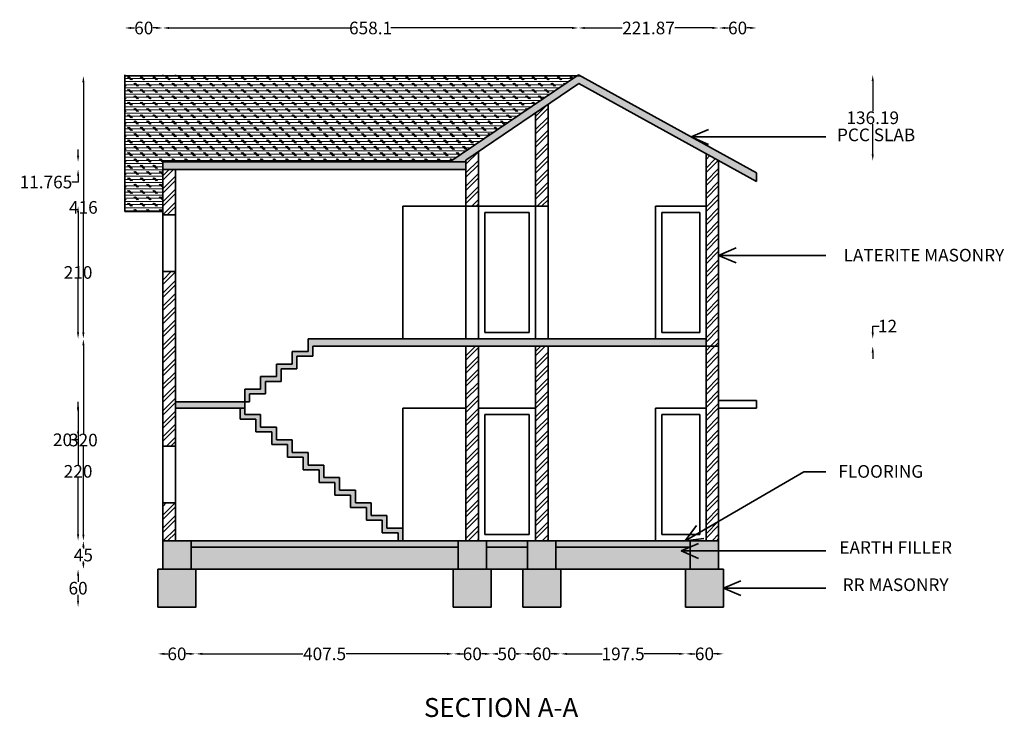
# Model space of a CAD drawing. Units: centimetres. Extents: x 10444 to 13814, y 8288 to 11191.
# Tile 7 of 9: x 12167 to 13725, y 8288 to 9393. Entities that reach past the tile are written whole.
import ezdxf

# ---------------------------------------------------------------- set-up
doc = ezdxf.new("R2010")
doc.units = ezdxf.units.CM
doc.header["$MEASUREMENT"] = 0
for name, color, linetype, lineweight in [('A-ANNO-DIMS', 2, 'Continuous', 18), ('A-ANNO-TEXT', 7, 'Continuous', 25), ('A-SECT', 7, 'Continuous', 35), ('A-SECT-PATT', 8, 'Continuous', 13)]:
    doc.layers.add(name, color=color, linetype=linetype, lineweight=lineweight)
doc.styles.get("Standard").update_dxf_attribs({"font": 'arial.ttf'})
doc.dimstyles.get("Standard").update_dxf_attribs({"dimtxt": 20, "dimasz": 10, "dimexe": 0.18, "dimexo": 0.0625, "dimgap": 0.09, "dimtad": 0, "dimtih": 1, "dimtoh": 1, "dimdec": 0, "dimzin": 0, "dimdsep": 46, "dimtxsty": 'Standard', "dimcen": 0.09, "dimse1": 1, "dimse2": 1, "dimadec": 0, "dimazin": 0, "dimtfac": 1, "dimtdec": 0, "dimtofl": 0, "dimtmove": 0, "dimatfit": 3, "dimfxl": 1, "dimtolj": 1, "dimtzin": 0, "dimarcsym": 0})

# ---------------------------------------------------------------- blocks, each defined once
blk = doc.blocks.new('*D23')
at = {"layer": 'A-ANNO-DIMS', "color": 0, "lineweight": -2, "transparency": 16777216}
for p, q in [((12267.5, 8557.5), (12267.5, 8555.3)), ((12267.5, 8532.6), (12267.5, 8534.8))]:
    blk.add_line(p, q, dxfattribs=at)
at = {"layer": 'A-ANNO-DIMS', "color": 0, "transparency": 16777216}
for points in [[(12265.8, 8557.5), (12269.2, 8557.5), (12267.5, 8567.5)], [(12265.8, 8532.6), (12269.2, 8532.6), (12267.5, 8522.6)]]:
    blk.add_solid(points, dxfattribs=at)
at = {"layer": 'Defpoints', "color": 0, "transparency": 16777216}
for p in [(12393.1, 8567.5), (12267.5, 8522.6), (12393.1, 8522.6)]:
    blk.add_point(p, dxfattribs=at)
at = {"layer": 'A-ANNO-DIMS', "color": 0, "transparency": 16777216, "insert": (12267.5, 8545), "char_height": 20, "attachment_point": 5}
blk.add_mtext('\\A1;45', dxfattribs=at)
blk = doc.blocks.new('*D24')
at = {"layer": 'A-ANNO-DIMS', "color": 0, "lineweight": -2, "transparency": 16777216}
for p, q in [((12267.5, 8877), (12267.5, 8737.6)), ((12267.5, 8577.5), (12267.5, 8716.9))]:
    blk.add_line(p, q, dxfattribs=at)
at = {"layer": 'A-ANNO-DIMS', "color": 0, "transparency": 16777216}
for points in [[(12265.8, 8877), (12269.2, 8877), (12267.5, 8887)], [(12265.8, 8577.5), (12269.2, 8577.5), (12267.5, 8567.5)]]:
    blk.add_solid(points, dxfattribs=at)
at = {"layer": 'Defpoints', "color": 0, "transparency": 16777216}
for p in [(12267.5, 8887), (12393.1, 8887), (12393.1, 8567.5)]:
    blk.add_point(p, dxfattribs=at)
at = {"layer": 'A-ANNO-DIMS', "color": 0, "transparency": 16777216, "insert": (12267.5, 8727.2), "char_height": 20, "attachment_point": 5}
blk.add_mtext('\\A1;320', dxfattribs=at)
blk = doc.blocks.new('*D25')
at = {"layer": 'A-ANNO-DIMS', "color": 0, "lineweight": -2, "transparency": 16777216}
for p, q in [((12267.5, 9293.8), (12267.5, 9106)), ((12267.5, 8897.6), (12267.5, 9085.4))]:
    blk.add_line(p, q, dxfattribs=at)
at = {"layer": 'A-ANNO-DIMS', "color": 0, "transparency": 16777216}
for points in [[(12265.8, 9293.8), (12269.2, 9293.8), (12267.5, 9303.8)], [(12265.8, 8897.6), (12269.2, 8897.6), (12267.5, 8887.6)]]:
    blk.add_solid(points, dxfattribs=at)
at = {"layer": 'Defpoints', "color": 0, "transparency": 16777216}
for p in [(12267.5, 9303.8), (12623.1, 9303.8), (12623.1, 8887.6)]:
    blk.add_point(p, dxfattribs=at)
at = {"layer": 'A-ANNO-DIMS', "color": 0, "transparency": 16777216, "insert": (12267.5, 9095.7), "char_height": 20, "attachment_point": 5}
blk.add_mtext('\\A1;416', dxfattribs=at)
blk = doc.blocks.new('*D107')
at = {"layer": 'A-ANNO-DIMS', "color": 0, "lineweight": -2, "transparency": 16777216}
for p, q in [((12343.1, 9379.8), (12348.6, 9379.8)), ((12383.1, 9379.8), (12377.5, 9379.8))]:
    blk.add_line(p, q, dxfattribs=at)
at = {"layer": 'A-ANNO-DIMS', "color": 0, "transparency": 16777216}
for points in [[(12343.1, 9381.5), (12343.1, 9378.2), (12333.1, 9379.8)], [(12383.1, 9381.5), (12383.1, 9378.2), (12393.1, 9379.8)]]:
    blk.add_solid(points, dxfattribs=at)
at = {"layer": 'Defpoints', "color": 0, "transparency": 16777216}
for p in [(12393.1, 9379.8), (12333.1, 9088.9), (12393.1, 9088.9)]:
    blk.add_point(p, dxfattribs=at)
at = {"layer": 'A-ANNO-DIMS', "color": 0, "transparency": 16777216, "insert": (12363.1, 9379.8), "char_height": 20, "attachment_point": 5}
blk.add_mtext('\\A1;60', dxfattribs=at)
blk = doc.blocks.new('*D108')
at = {"layer": 'A-ANNO-DIMS', "color": 0, "lineweight": -2, "transparency": 16777216}
for p, q in [((12403.1, 9379.8), (12690.2, 9379.8)), ((13041.2, 9379.8), (12754.1, 9379.8))]:
    blk.add_line(p, q, dxfattribs=at)
at = {"layer": 'A-ANNO-DIMS', "color": 0, "transparency": 16777216}
for points in [[(12403.1, 9381.5), (12403.1, 9378.2), (12393.1, 9379.8)], [(13041.2, 9381.5), (13041.2, 9378.2), (13051.2, 9379.8)]]:
    blk.add_solid(points, dxfattribs=at)
at = {"layer": 'Defpoints', "color": 0, "transparency": 16777216}
for p in [(13051.2, 9379.8), (13051.2, 9305.7), (12393.1, 9167.6)]:
    blk.add_point(p, dxfattribs=at)
at = {"layer": 'A-ANNO-DIMS', "color": 0, "transparency": 16777216, "insert": (12722.1, 9379.8), "char_height": 20, "attachment_point": 5}
blk.add_mtext('\\A1;658.1', dxfattribs=at)
blk = doc.blocks.new('*D109')
at = {"layer": 'A-ANNO-DIMS', "color": 0, "lineweight": -2, "transparency": 16777216}
for p, q in [((13061.2, 9379.8), (13120.4, 9379.8)), ((13263.1, 9379.8), (13203.9, 9379.8))]:
    blk.add_line(p, q, dxfattribs=at)
at = {"layer": 'A-ANNO-DIMS', "color": 0, "transparency": 16777216}
for points in [[(13061.2, 9381.5), (13061.2, 9378.2), (13051.2, 9379.8)], [(13263.1, 9381.5), (13263.1, 9378.2), (13273.1, 9379.8)]]:
    blk.add_solid(points, dxfattribs=at)
at = {"layer": 'Defpoints', "color": 0, "transparency": 16777216}
for p in [(13273.1, 9379.8), (13051.2, 9305.7), (13273.1, 9169.5)]:
    blk.add_point(p, dxfattribs=at)
at = {"layer": 'A-ANNO-DIMS', "color": 0, "transparency": 16777216, "insert": (13162.1, 9379.8), "char_height": 20, "attachment_point": 5}
blk.add_mtext('\\A1;221.87', dxfattribs=at)
blk = doc.blocks.new('*D110')
at = {"layer": 'A-ANNO-DIMS', "color": 0, "lineweight": -2, "transparency": 16777216}
for p, q in [((13283.1, 9379.8), (13288.6, 9379.8)), ((13323.1, 9379.8), (13317.5, 9379.8))]:
    blk.add_line(p, q, dxfattribs=at)
at = {"layer": 'A-ANNO-DIMS', "color": 0, "transparency": 16777216}
for points in [[(13283.1, 9381.5), (13283.1, 9378.2), (13273.1, 9379.8)], [(13323.1, 9381.5), (13323.1, 9378.2), (13333.1, 9379.8)]]:
    blk.add_solid(points, dxfattribs=at)
at = {"layer": 'Defpoints', "color": 0, "transparency": 16777216}
for p in [(13333.1, 9379.8), (13273.1, 9169.5), (13333.1, 9136.4)]:
    blk.add_point(p, dxfattribs=at)
at = {"layer": 'A-ANNO-DIMS', "color": 0, "transparency": 16777216, "insert": (13303.1, 9379.8), "char_height": 20, "attachment_point": 5}
blk.add_mtext('\\A1;60', dxfattribs=at)
blk = doc.blocks.new('*D111')
at = {"layer": 'A-ANNO-DIMS', "color": 0, "lineweight": -2, "transparency": 16777216}
for p, q in [((12395.6, 8388.5), (12401.1, 8388.5)), ((12435.6, 8388.5), (12430, 8388.5))]:
    blk.add_line(p, q, dxfattribs=at)
at = {"layer": 'A-ANNO-DIMS', "color": 0, "transparency": 16777216}
for points in [[(12395.6, 8390.2), (12395.6, 8386.8), (12385.6, 8388.5)], [(12435.6, 8390.2), (12435.6, 8386.8), (12445.6, 8388.5)]]:
    blk.add_solid(points, dxfattribs=at)
at = {"layer": 'Defpoints', "color": 0, "transparency": 16777216}
for p in [(12385.6, 8462.5), (12445.6, 8462.5), (12445.6, 8388.5)]:
    blk.add_point(p, dxfattribs=at)
at = {"layer": 'A-ANNO-DIMS', "color": 0, "transparency": 16777216, "insert": (12415.6, 8388.5), "char_height": 20, "attachment_point": 5}
blk.add_mtext('\\A1;60', dxfattribs=at)
blk = doc.blocks.new('*D112')
at = {"layer": 'A-ANNO-DIMS', "color": 0, "lineweight": -2, "transparency": 16777216}
for p, q in [((12455.6, 8388.5), (12615, 8388.5)), ((12843.1, 8388.5), (12683.6, 8388.5))]:
    blk.add_line(p, q, dxfattribs=at)
at = {"layer": 'A-ANNO-DIMS', "color": 0, "transparency": 16777216}
for points in [[(12455.6, 8390.2), (12455.6, 8386.8), (12445.6, 8388.5)], [(12843.1, 8390.2), (12843.1, 8386.8), (12853.1, 8388.5)]]:
    blk.add_solid(points, dxfattribs=at)
at = {"layer": 'Defpoints', "color": 0, "transparency": 16777216}
for p in [(12445.6, 8462.5), (12853.1, 8462.6), (12853.1, 8388.5)]:
    blk.add_point(p, dxfattribs=at)
at = {"layer": 'A-ANNO-DIMS', "color": 0, "transparency": 16777216, "insert": (12649.3, 8388.5), "char_height": 20, "attachment_point": 5}
blk.add_mtext('\\A1;407.5', dxfattribs=at)
blk = doc.blocks.new('*D113')
at = {"layer": 'A-ANNO-DIMS', "color": 0, "lineweight": -2, "transparency": 16777216}
for p, q in [((12863.1, 8388.5), (12868.6, 8388.5)), ((12903.1, 8388.5), (12897.5, 8388.5))]:
    blk.add_line(p, q, dxfattribs=at)
at = {"layer": 'A-ANNO-DIMS', "color": 0, "transparency": 16777216}
for points in [[(12863.1, 8390.2), (12863.1, 8386.8), (12853.1, 8388.5)], [(12903.1, 8390.2), (12903.1, 8386.8), (12913.1, 8388.5)]]:
    blk.add_solid(points, dxfattribs=at)
at = {"layer": 'Defpoints', "color": 0, "transparency": 16777216}
for p in [(12853.1, 8462.6), (12913.1, 8462.6), (12913.1, 8388.5)]:
    blk.add_point(p, dxfattribs=at)
at = {"layer": 'A-ANNO-DIMS', "color": 0, "transparency": 16777216, "insert": (12883.1, 8388.5), "char_height": 20, "attachment_point": 5}
blk.add_mtext('\\A1;60', dxfattribs=at)
blk = doc.blocks.new('*D114')
at = {"layer": 'A-ANNO-DIMS', "color": 0, "lineweight": -2, "transparency": 16777216}
for p, q in [((12923.1, 8388.5), (12923.7, 8388.5)), ((12953.1, 8388.5), (12952.5, 8388.5))]:
    blk.add_line(p, q, dxfattribs=at)
at = {"layer": 'A-ANNO-DIMS', "color": 0, "transparency": 16777216}
for points in [[(12923.1, 8390.2), (12923.1, 8386.8), (12913.1, 8388.5)], [(12953.1, 8390.2), (12953.1, 8386.8), (12963.1, 8388.5)]]:
    blk.add_solid(points, dxfattribs=at)
at = {"layer": 'Defpoints', "color": 0, "transparency": 16777216}
for p in [(12913.1, 8462.6), (12963.1, 8462.6), (12963.1, 8388.5)]:
    blk.add_point(p, dxfattribs=at)
at = {"layer": 'A-ANNO-DIMS', "color": 0, "transparency": 16777216, "insert": (12938.1, 8388.5), "char_height": 20, "attachment_point": 5}
blk.add_mtext('\\A1;50', dxfattribs=at)
blk = doc.blocks.new('*D115')
at = {"layer": 'A-ANNO-DIMS', "color": 0, "lineweight": -2, "transparency": 16777216}
for p, q in [((12973.1, 8388.5), (12978.6, 8388.5)), ((13013.1, 8388.5), (13007.5, 8388.5))]:
    blk.add_line(p, q, dxfattribs=at)
at = {"layer": 'A-ANNO-DIMS', "color": 0, "transparency": 16777216}
for points in [[(12973.1, 8390.2), (12973.1, 8386.8), (12963.1, 8388.5)], [(13013.1, 8390.2), (13013.1, 8386.8), (13023.1, 8388.5)]]:
    blk.add_solid(points, dxfattribs=at)
at = {"layer": 'Defpoints', "color": 0, "transparency": 16777216}
for p in [(12963.1, 8462.6), (13023.1, 8462.6), (13023.1, 8388.5)]:
    blk.add_point(p, dxfattribs=at)
at = {"layer": 'A-ANNO-DIMS', "color": 0, "transparency": 16777216, "insert": (12993.1, 8388.5), "char_height": 20, "attachment_point": 5}
blk.add_mtext('\\A1;60', dxfattribs=at)
blk = doc.blocks.new('*D116')
at = {"layer": 'A-ANNO-DIMS', "color": 0, "lineweight": -2, "transparency": 16777216}
for p, q in [((13033.1, 8388.5), (13088.9, 8388.5)), ((13210.6, 8388.5), (13154.8, 8388.5))]:
    blk.add_line(p, q, dxfattribs=at)
at = {"layer": 'A-ANNO-DIMS', "color": 0, "transparency": 16777216}
for points in [[(13033.1, 8390.2), (13033.1, 8386.8), (13023.1, 8388.5)], [(13210.6, 8390.2), (13210.6, 8386.8), (13220.6, 8388.5)]]:
    blk.add_solid(points, dxfattribs=at)
at = {"layer": 'Defpoints', "color": 0, "transparency": 16777216}
for p in [(13023.1, 8462.6), (13220.6, 8462.6), (13220.6, 8388.5)]:
    blk.add_point(p, dxfattribs=at)
at = {"layer": 'A-ANNO-DIMS', "color": 0, "transparency": 16777216, "insert": (13121.8, 8388.5), "char_height": 20, "attachment_point": 5}
blk.add_mtext('\\A1;197.5', dxfattribs=at)
blk = doc.blocks.new('*D117')
at = {"layer": 'A-ANNO-DIMS', "color": 0, "lineweight": -2, "transparency": 16777216}
for p, q in [((13230.6, 8388.5), (13236.1, 8388.5)), ((13270.6, 8388.5), (13265, 8388.5))]:
    blk.add_line(p, q, dxfattribs=at)
at = {"layer": 'A-ANNO-DIMS', "color": 0, "transparency": 16777216}
for points in [[(13230.6, 8390.2), (13230.6, 8386.8), (13220.6, 8388.5)], [(13270.6, 8390.2), (13270.6, 8386.8), (13280.6, 8388.5)]]:
    blk.add_solid(points, dxfattribs=at)
at = {"layer": 'Defpoints', "color": 0, "transparency": 16777216}
for p in [(13220.6, 8462.6), (13280.6, 8462.6), (13280.6, 8388.5)]:
    blk.add_point(p, dxfattribs=at)
at = {"layer": 'A-ANNO-DIMS', "color": 0, "transparency": 16777216, "insert": (13250.6, 8388.5), "char_height": 20, "attachment_point": 5}
blk.add_mtext('\\A1;60', dxfattribs=at)
blk = doc.blocks.new('*D118')
at = {"layer": 'A-ANNO-DIMS', "color": 0, "lineweight": -2, "transparency": 16777216}
for p, q in [((12259.1, 8512.5), (12259.1, 8502.8)), ((12259.1, 8472.5), (12259.1, 8482.2))]:
    blk.add_line(p, q, dxfattribs=at)
at = {"layer": 'A-ANNO-DIMS', "color": 0, "transparency": 16777216}
for points in [[(12257.4, 8512.5), (12260.7, 8512.5), (12259.1, 8522.5)], [(12257.4, 8472.5), (12260.7, 8472.5), (12259.1, 8462.5)]]:
    blk.add_solid(points, dxfattribs=at)
at = {"layer": 'Defpoints', "color": 0, "transparency": 16777216}
for p in [(12259.1, 8522.5), (12385.6, 8522.5), (12385.6, 8462.5)]:
    blk.add_point(p, dxfattribs=at)
at = {"layer": 'A-ANNO-DIMS', "color": 0, "transparency": 16777216, "insert": (12259.1, 8492.5), "char_height": 20, "attachment_point": 5}
blk.add_mtext('\\A1;60', dxfattribs=at)
blk = doc.blocks.new('*D119')
at = {"layer": 'A-ANNO-DIMS', "color": 0, "lineweight": -2, "transparency": 16777216}
for p, q in [((12259.1, 8777.6), (12259.1, 8687.9)), ((12259.1, 8577.6), (12259.1, 8667.3))]:
    blk.add_line(p, q, dxfattribs=at)
at = {"layer": 'A-ANNO-DIMS', "color": 0, "transparency": 16777216}
for points in [[(12257.4, 8777.6), (12260.7, 8777.6), (12259.1, 8787.6)], [(12257.4, 8577.6), (12260.7, 8577.6), (12259.1, 8567.6)]]:
    blk.add_solid(points, dxfattribs=at)
at = {"layer": 'Defpoints', "color": 0, "transparency": 16777216}
for p in [(12259.1, 8787.6), (12413.1, 8787.6), (12413.1, 8567.6)]:
    blk.add_point(p, dxfattribs=at)
at = {"layer": 'A-ANNO-DIMS', "color": 0, "transparency": 16777216, "insert": (12259.1, 8677.6), "char_height": 20, "attachment_point": 5}
blk.add_mtext('\\A1;220', dxfattribs=at)
blk = doc.blocks.new('*D120')
at = {"layer": 'A-ANNO-DIMS', "color": 0, "lineweight": -2, "transparency": 16777216}
for p, q in [((12259.1, 9087.6), (12259.1, 9002.9)), ((12259.1, 8897.6), (12259.1, 8982.3))]:
    blk.add_line(p, q, dxfattribs=at)
at = {"layer": 'A-ANNO-DIMS', "color": 0, "transparency": 16777216}
for points in [[(12257.4, 9087.6), (12260.7, 9087.6), (12259.1, 9097.6)], [(12257.4, 8897.6), (12260.7, 8897.6), (12259.1, 8887.6)]]:
    blk.add_solid(points, dxfattribs=at)
at = {"layer": 'Defpoints', "color": 0, "transparency": 16777216}
for p in [(12259.1, 9097.6), (12773.1, 9097.6), (12773.1, 8887.6)]:
    blk.add_point(p, dxfattribs=at)
at = {"layer": 'A-ANNO-DIMS', "color": 0, "transparency": 16777216, "insert": (12259.1, 8992.6), "char_height": 20, "attachment_point": 5}
blk.add_mtext('\\A1;210', dxfattribs=at)
blk = doc.blocks.new('*D121')
at = {"layer": 'A-ANNO-DIMS', "color": 0, "lineweight": -2, "transparency": 16777216}
for p, q in [((12259.1, 9177.6), (12259.1, 9187.6)), ((12259.1, 9135.8), (12249.1, 9135.8)), ((12259.1, 9145.8), (12259.1, 9135.8))]:
    blk.add_line(p, q, dxfattribs=at)
at = {"layer": 'A-ANNO-DIMS', "color": 0, "transparency": 16777216}
for points in [[(12257.4, 9177.6), (12260.7, 9177.6), (12259.1, 9167.6)], [(12257.4, 9145.8), (12260.7, 9145.8), (12259.1, 9155.8)]]:
    blk.add_solid(points, dxfattribs=at)
at = {"layer": 'Defpoints', "color": 0, "transparency": 16777216}
for p in [(12393.1, 9167.6), (12259.1, 9155.8), (12413.1, 9155.8)]:
    blk.add_point(p, dxfattribs=at)
at = {"layer": 'A-ANNO-DIMS', "color": 0, "transparency": 16777216, "insert": (12208.3, 9135.8), "char_height": 20, "attachment_point": 5}
blk.add_mtext('\\A1;11.765', dxfattribs=at)
blk = doc.blocks.new('*D122')
at = {"layer": 'A-ANNO-DIMS', "color": 0, "lineweight": -2, "transparency": 16777216}
for p, q in [((13517, 8897.6), (13517, 8907.6)), ((13517, 8907.6), (13527, 8907.6)), ((13517, 8865.6), (13517, 8855.6))]:
    blk.add_line(p, q, dxfattribs=at)
at = {"layer": 'A-ANNO-DIMS', "color": 0, "transparency": 16777216}
for points in [[(13515.3, 8897.6), (13518.7, 8897.6), (13517, 8887.6)], [(13515.3, 8865.6), (13518.7, 8865.6), (13517, 8875.6)]]:
    blk.add_solid(points, dxfattribs=at)
at = {"layer": 'Defpoints', "color": 0, "transparency": 16777216}
for p in [(13253.1, 8887.6), (13517, 8887.6), (13253.1, 8875.6)]:
    blk.add_point(p, dxfattribs=at)
at = {"layer": 'A-ANNO-DIMS', "color": 0, "transparency": 16777216, "insert": (13540.4, 8907.6), "char_height": 20, "attachment_point": 5}
blk.add_mtext('\\A1;12', dxfattribs=at)
blk = doc.blocks.new('*D123')
at = {"layer": 'A-ANNO-DIMS', "color": 0, "lineweight": -2, "transparency": 16777216}
for p, q in [((13517, 9295.7), (13517, 9247.9)), ((13517, 9179.5), (13517, 9227.3))]:
    blk.add_line(p, q, dxfattribs=at)
at = {"layer": 'A-ANNO-DIMS', "color": 0, "transparency": 16777216}
for points in [[(13515.3, 9295.7), (13518.7, 9295.7), (13517, 9305.7)], [(13515.3, 9179.5), (13518.7, 9179.5), (13517, 9169.5)]]:
    blk.add_solid(points, dxfattribs=at)
at = {"layer": 'Defpoints', "color": 0, "transparency": 16777216}
for p in [(13051.2, 9305.7), (13517, 9305.7), (13273.1, 9169.5)]:
    blk.add_point(p, dxfattribs=at)
at = {"layer": 'A-ANNO-DIMS', "color": 0, "transparency": 16777216, "insert": (13517, 9237.6), "char_height": 20, "attachment_point": 5}
blk.add_mtext('\\A1;136.19', dxfattribs=at)
blk = doc.blocks.new('*D124')
at = {"layer": 'A-ANNO-DIMS', "color": 0, "lineweight": -2, "transparency": 16777216}
for p, q in [((12259.1, 8777.6), (12259.1, 8787.6)), ((12259.1, 8737.6), (12259.1, 8727.6)), ((12259.1, 8727.6), (12249.1, 8727.6))]:
    blk.add_line(p, q, dxfattribs=at)
at = {"layer": 'A-ANNO-DIMS', "color": 0, "transparency": 16777216}
for points in [[(12257.4, 8777.6), (12260.7, 8777.6), (12259.1, 8767.6)], [(12257.4, 8737.6), (12260.7, 8737.6), (12259.1, 8747.6)]]:
    blk.add_solid(points, dxfattribs=at)
at = {"layer": 'Defpoints', "color": 0, "transparency": 16777216}
for p in [(12548.1, 8767.6), (12259.1, 8747.6), (12573.1, 8747.6)]:
    blk.add_point(p, dxfattribs=at)
at = {"layer": 'A-ANNO-DIMS', "color": 0, "transparency": 16777216, "insert": (12234.5, 8727.6), "char_height": 20, "attachment_point": 5}
blk.add_mtext('\\A1;20', dxfattribs=at)

msp = doc.modelspace()

# ---------------------------------------------------------------- hatches: boundary and pattern name
at = {"layer": 'A-SECT-PATT'}
h = msp.add_hatch(dxfattribs=at)
h.set_pattern_fill('CORK', color=256, scale=40)
h.set_pattern_definition([(0, (0, 0), (0, 5), []), (135, (2.5, -2.5), (-10, -10), [7.071068, -7.071068]), (135, (3.75, -2.5), (-10, -10), [7.071068, -7.071068]), (135, (5, -2.5), (-10, -10), [7.071068, -7.071068])])
h.paths.add_polyline_path([(13048.419, 9303.8312), (12333.077, 9303.8312), (12333.077, 9088.8963), (12393.077, 9088.8963), (12393.077, 9167.5959), (12847.6732, 9167.5959)])
h = msp.add_hatch(dxfattribs=at)
h.set_pattern_fill('AR-SAND', color=256, scale=5)
h.set_pattern_definition([(37.5, (0, 0), (-0.3149668, 9.634119), [0, -7.6, 0, -8.5, 0, -8.125]), (7.5, (0, 0), (8.848884, 14.11073), [0, -4.1, 0, -6.85, 0, -2.625]), (327.5, (-6.15, 0), (15.5707093, 0.0282953), [0, -2.5, 0, -9, 0, -11.75]), (317.5, (-6.15, 0), (15.030633, 4.388378), [0, -1.25, 0, -5.9, 0, -6.75])])
h.paths.add_polyline_path([(13051.8537, 9291.6597), (13333.077, 9136.4165), (13333.077, 9150.1235), (13054.6352, 9303.8312), (13048.419, 9303.8312), (12847.6732, 9167.5959), (12873.077, 9167.5959), (12873.077, 9170.3336)])
h.paths.add_polyline_path([(12873.077, 9167.5959), (12847.6732, 9167.5959), (12393.077, 9167.5959), (12393.077, 9155.8312), (12873.077, 9155.8312)])
h.paths.add_polyline_path([(13253.077, 8887.5959), (12873.077, 8887.5959), (12623.077, 8887.5959), (12623.077, 8867.5959), (12598.077, 8867.5959), (12598.077, 8847.5959), (12573.077, 8847.5959), (12573.077, 8827.5959), (12548.077, 8827.5959), (12548.077, 8807.5959), (12523.077, 8807.5959), (12523.077, 8787.5959), (12530.577, 8787.5959), (12530.577, 8800.0959), (12555.577, 8800.0959), (12555.577, 8820.0959), (12580.577, 8820.0959), (12580.577, 8840.0959), (12605.577, 8840.0959), (12605.577, 8860.0959), (12630.577, 8860.0959), (12630.577, 8875.5959), (13253.077, 8875.5959)])
h.paths.add_polyline_path([(12523.077, 8787.5959), (12413.077, 8787.5959), (12413.077, 8777.5959), (12523.077, 8777.5959)])
h.paths.add_polyline_path([(12548.077, 8767.5959), (12523.077, 8767.5959), (12523.077, 8777.5959), (12515.577, 8777.5959), (12515.577, 8760.0959), (12540.577, 8760.0959), (12540.577, 8740.0959), (12565.577, 8740.0959), (12565.577, 8720.0959), (12590.577, 8720.0959), (12590.577, 8700.0959), (12615.577, 8700.0959), (12615.577, 8680.0959), (12640.577, 8680.0959), (12640.577, 8660.0959), (12665.577, 8660.0959), (12665.577, 8640.0959), (12690.577, 8640.0959), (12690.577, 8620.0959), (12715.577, 8620.0959), (12715.577, 8600.0959), (12740.577, 8600.0959), (12740.577, 8580.0959), (12765.577, 8580.0959), (12765.577, 8567.5959), (12773.077, 8567.5959), (12773.077, 8587.5959), (12748.077, 8587.5959), (12748.077, 8607.5959), (12723.077, 8607.5959), (12723.077, 8627.5959), (12698.077, 8627.5959), (12698.077, 8647.5959), (12673.077, 8647.5959), (12673.077, 8667.5959), (12648.077, 8667.5959), (12648.077, 8687.5959), (12623.077, 8687.5959), (12623.077, 8707.5959), (12598.077, 8707.5959), (12598.077, 8727.5959), (12573.077, 8727.5959), (12573.077, 8747.5959), (12548.077, 8747.5959)])
h.paths.add_polyline_path([(12860.577, 8567.5959), (12438.077, 8567.5959), (12438.077, 8557.5959), (12860.577, 8557.5959)])
h.paths.add_polyline_path([(12970.577, 8567.5959), (12905.577, 8567.5959), (12905.577, 8557.5959), (12970.577, 8557.5959)])
h.paths.add_polyline_path([(13228.077, 8567.5959), (13015.577, 8567.5959), (13015.577, 8557.5959), (13228.077, 8557.5959)])
h.paths.add_polyline_path([(12860.577, 8557.5959), (12438.077, 8557.5959), (12438.077, 8522.5959), (12860.577, 8522.5959)])
h.paths.add_polyline_path([(12970.577, 8557.5959), (12905.577, 8557.5959), (12905.577, 8522.5959), (12970.577, 8522.5959)])
h.paths.add_polyline_path([(13228.077, 8557.5959), (13015.577, 8557.5959), (13015.577, 8522.5959), (13023.077, 8522.5959), (13228.077, 8522.5959)])
h = msp.add_hatch(dxfattribs=at)
h.set_pattern_fill('AR-CONC', color=256, scale=20)
h.set_pattern_definition([(50, (0, 0), (143.452, -12.5504), [15, -165]), (355, (0, 0), (-27.7503, 150.4384), [12, -132]), (100.4514, (11.95, -1.05), (115.7018, 137.888), [12.748, -140.2284]), (46.1842, (0, 40), (213.4483, -33.1039), [22.5, -247.5]), (96.6356, (17.79, 37.24), (186.9324, 194.8237), [19.122, -210.3428]), (351.1842, (0, 40), (186.9324, 194.8237), [18, -198]), (21, (20, 30), (119.3814, -80.5238), [15, -165]), (326, (20, 30), (48.663, 145.03), [12, -132]), (71.4514, (29.95, 23.29), (168.0445, 64.5062), [12.748, -140.2284]), (37.5, (0, 0), (2.43197, 66.57877), [0, -130.4, 0, -134, 0, -132.5]), (7.5, (0, 0), (52.6139, 78.88234), [0, -76.4, 0, -127.4, 0, -50.5]), (327.5, (-44.6, 0), (106.76449, -4.51097), [0, -50, 0, -156, 0, -207]), (317.5, (-64.6, 0), (116.63723, 20.021), [0, -65, 0, -103.6, 0, -147])])
h.paths.add_polyline_path([(13051.8537, 9291.6597), (13333.077, 9136.4165), (13333.077, 9150.1235), (13054.6352, 9303.8312), (13048.419, 9303.8312), (12847.6732, 9167.5959), (12873.077, 9167.5959), (12873.077, 9170.3336)])
h = msp.add_hatch(dxfattribs=at)
h.set_pattern_fill('ANSI32', color=256, scale=39)
h.paths.add_polyline_path([(12413.077, 9155.8312), (12393.077, 9155.8312), (12393.077, 9084), (12413.077, 9084)])
h.paths.add_polyline_path([(12413.077, 8994), (12393.077, 8994), (12393.077, 8717.5959), (12413.077, 8717.5959)])
h.paths.add_polyline_path([(12413.077, 8627.5959), (12393.077, 8627.5959), (12393.077, 8567.5), (12413.077, 8567.5)])
h.paths.add_polyline_path([(12893.077, 9183.9066), (12873.077, 9170.3336), (12873.077, 9097.5959), (12893.077, 9097.5959)])
h.paths.add_polyline_path([(13003.077, 9258.5576), (12983.077, 9244.9847), (12983.077, 9097.5959), (13003.077, 9097.5959)])
h = msp.add_hatch(dxfattribs=at)
h.set_pattern_fill('ANSI32', color=256, scale=39)
h.paths.add_polyline_path([(13273.077, 9169.5382), (13253.077, 9180.5788), (13253.077, 8875.5959), (13273.077, 8875.5959)])
h = msp.add_hatch(dxfattribs=at)
h.set_pattern_fill('ANSI32', color=256, scale=39)
h.paths.add_polyline_path([(13273.077, 8875.5959), (13253.077, 8875.5959), (13253.077, 8567.5959), (13273.077, 8567.5959)])
h.paths.add_polyline_path([(13003.077, 8875.5959), (12983.077, 8875.5959), (12983.077, 8567.5959), (13003.077, 8567.5959)])
h.paths.add_polyline_path([(12893.077, 8875.5959), (12873.077, 8875.5959), (12873.077, 8567.5959), (12893.077, 8567.5959)])
h = msp.add_hatch(dxfattribs=at)
h.set_pattern_fill('GRAVEL', color=256, scale=40)
h.set_pattern_definition([(228.012788, (28.8, 40), (-320, -360), [5.38144, -532.76352]), (184.969741, (25.2, 36), (480, 40), [9.23472, -914.23699]), (132.510447, (16, 35.2), (400, -440), [6.51152, -644.6413]), (267.273689, (0.4, 25.2), (40, 800), [8.40952, -832.54232]), (292.833654, (0, 16.8), (-200, 480), [8.2462, -816.374925]), (357.273689, (3.2, 9.2), (-800, 40), [8.40952, -832.54232]), (37.69424, (11.6, 8.8), (-520, -400), [11.12116, -1100.99394]), (72.255328, (20.4, 15.6), (280, 880), [10.49952, -1039.45286]), (121.429566, (23.6, 25.6), (-320, 520), [8.438, -835.36292]), (175.236358, (19.2, 32.8), (440, -40), [9.63328, -472.0305]), (222.397438, (9.6, 33.6), (-480, -440), [12.45792, -1233.335]), (138.814075, (40, 24.8), (-280, 240), [4.25204, -420.95379]), (171.469234, (36.8, 27.6), (520, -80), [8.08948, -800.86046]), (225, (28.8, 28.8), (-4e-15, -40), [5.65684, -50.9117]), (203.19859, (26, 33.6), (200, 80), [3.04632, -301.5846]), (291.80141, (23.2, 32.4), (-40, 120), [4.30812, -211.09847]), (30.963757, (24.8, 28.4), (120, 80), [6.99716, -226.24092]), (161.56505, (30.8, 32), (80, -40), [5.05964, -121.43147]), (16.38954, (0, 32.4), (400, 120), [7.088, -701.71381]), (70.346176, (6.8, 34.4), (-160, -440), [5.94644, -588.69631]), (293.19859, (30.8, 40), (-80, 200), [6.0926, -298.53832]), (343.61046, (33.2, 34.4), (-400, 120), [7.088, -701.71381]), (339.443955, (0, 7.6), (-200, 80), [6.8352, -334.92495]), (294.77514, (6.4, 5.2), (-200, 440), [5.72712, -566.98572]), (66.80141, (31.2, 0), (80, 200), [6.0926, -298.53832]), (17.354025, (33.6, 5.6), (-520, -160), [6.70524, -663.81694]), (69.443955, (11.6, 0), (-80, -200), [3.4176, -338.34255]), (101.30993, (28.8, 0), (-40, 160), [2.0396, -201.92118]), (165.96376, (28.4, 2), (120, -40), [8.2462, -156.67803]), (186.009006, (20.4, 4), (400, 40), [7.642, -756.55693]), (303.69007, (24.8, 24.8), (-40, 80), [5.76888, -138.45317]), (353.157227, (28, 20), (680, -80), [10.07176, -997.102505]), (60.945396, (38, 18.8), (-160, -280), [4.11824, -407.70697]), (90, (40, 22.4), (-40, 40), [2.4, -37.6]), (120.256437, (19.6, 5.2), (160, -280), [5.55696, -550.1408]), (48.012788, (16.8, 10), (320, 360), [10.76288, -527.38208]), (0, (24, 18), (40, 40), [10.4, -29.6]), (325.304846, (34.4, 18), (400, -280), [6.32456, -626.13097]), (254.054604, (39.6, 14.4), (-40, -160), [5.82408, -285.38032]), (207.645975, (38, 8.8), (-760, -400), [9.4826, -938.77897]), (175.426079, (29.6, 4.4), (-520, 40), [10.03196, -993.16294])])
h.paths.add_polyline_path([(12445.577, 8522.5), (12385.577, 8522.5), (12385.577, 8462.5), (12445.577, 8462.5)])
h.paths.add_polyline_path([(12438.077, 8567.5), (12393.077, 8567.5), (12393.077, 8522.5959), (12438.077, 8522.5959)])
h.paths.add_polyline_path([(12905.577, 8567.5959), (12860.577, 8567.5959), (12860.577, 8522.5959), (12905.577, 8522.5959)])
h.paths.add_polyline_path([(12913.077, 8522.5959), (12853.077, 8522.5959), (12853.077, 8462.5959), (12913.077, 8462.5959)])
h.paths.add_polyline_path([(13023.077, 8522.5959), (12963.077, 8522.5959), (12963.077, 8462.5959), (13023.077, 8462.5959)])
h.paths.add_polyline_path([(13015.577, 8567.5959), (12970.577, 8567.5959), (12970.577, 8522.5959), (13015.577, 8522.5959)])
h.paths.add_polyline_path([(13273.077, 8567.5959), (13228.077, 8567.5959), (13228.077, 8522.5959), (13273.077, 8522.5959)])
h.paths.add_polyline_path([(13280.577, 8522.5959), (13220.577, 8522.5959), (13220.577, 8462.5959), (13280.577, 8462.5959)])

# ---------------------------------------------------------------- linework, layer by layer
at = {"layer": 'A-SECT'}
for p, q in [((12333.077, 9305.8312), (12333.077, 9088.8963)), ((12393.077, 9305.8312), (12393.077, 9303.8312)), ((12413.077, 9305.8312), (12413.077, 9303.8312)), ((12847.6732, 9167.5959), (13051.2073, 9305.7235)), ((13051.2073, 9305.7235), (13333.077, 9150.1235)), ((12333.077, 9303.8312), (13054.6352, 9303.8312)), ((12873.077, 9170.3336), (13051.8537, 9291.6597)), ((13051.8537, 9291.6597), (13333.077, 9136.4165)), ((13003.077, 8887.5959), (13003.077, 9258.5576)), ((12983.077, 8887.5959), (12983.077, 9244.9847)), ((13229.7591, 9207.1579), (13257.2591, 9218.9959)), ((13443, 9207.1579), (13229.7591, 9207.1579)), ((13229.7591, 9207.1579), (13257.2591, 9195.3199)), ((12893.077, 8887.5959), (12893.077, 9183.9066)), ((13253.077, 8875.5959), (13253.077, 9180.5788)), ((12393.077, 9167.5959), (12873.077, 9167.5959)), ((12393.077, 9167.5959), (12393.077, 8522.5)), ((12873.077, 8887.5959), (12873.077, 9170.3336)), ((13273.077, 8557.5959), (13273.077, 9169.5382)), ((12393.077, 9155.8312), (12873.077, 9155.8312)), ((12413.077, 9155.8312), (12413.077, 8567.5959)), ((13333.077, 9150.1235), (13333.077, 9136.4165)), ((12333.077, 9088.8963), (12393.077, 9088.8963)), ((12773.077, 9097.5959), (12873.077, 9097.5959)), ((12773.077, 9097.5959), (12773.077, 8887.5959)), ((12873.077, 9097.5959), (13003.077, 9097.5959)), ((12903.077, 9087.5959), (12973.077, 9087.5959)), ((12903.077, 8897.5959), (12903.077, 9087.5959)), ((12973.077, 8897.5959), (12973.077, 9087.5959)), ((13173.077, 9097.5959), (13173.077, 8887.5959)), ((13173.077, 9097.5959), (13253.077, 9097.5959)), ((13183.077, 9087.5959), (13183.077, 8897.5959)), ((13183.077, 9087.5959), (13243.077, 9087.5959)), ((13243.077, 8897.5959), (13243.077, 9087.5959)), ((12393.077, 8994), (12393.077, 9084)), ((12393.077, 9084), (12413.077, 9084)), ((13273.077, 9019.5), (13300.577, 9031.338)), ((13443, 9019.5), (13273.077, 9019.5)), ((13273.077, 9019.5), (13300.577, 9007.662)), ((12413.077, 8994), (12393.077, 8994)), ((12623.077, 8887.5959), (12623.077, 8867.5959)), ((12623.077, 8887.5959), (12873.077, 8887.5959)), ((12873.077, 8887.5959), (13253.077, 8887.5959)), ((12903.077, 8897.5959), (12973.077, 8897.5959)), ((13183.077, 8897.5959), (13243.077, 8897.5959)), ((12630.577, 8875.5959), (12630.577, 8860.0959)), ((12630.577, 8875.5959), (13273.077, 8875.5959)), ((12873.077, 8875.5959), (12873.077, 8567.5959)), ((12893.077, 8875.5959), (12893.077, 8567.5959)), ((12983.077, 8875.5959), (12983.077, 8567.5959)), ((13003.077, 8875.5959), (13003.077, 8567.5959)), ((13253.077, 8567.5959), (13253.077, 8875.5959)), ((12598.077, 8867.5959), (12623.077, 8867.5959)), ((12598.077, 8867.5959), (12598.077, 8847.5959)), ((12605.577, 8860.0959), (12605.577, 8840.0959)), ((12605.577, 8860.0959), (12630.577, 8860.0959)), ((12573.077, 8847.5959), (12598.077, 8847.5959)), ((12573.077, 8847.5959), (12573.077, 8827.5959)), ((12580.577, 8840.0959), (12580.577, 8820.0959)), ((12580.577, 8840.0959), (12605.577, 8840.0959)), ((12548.077, 8827.5959), (12573.077, 8827.5959)), ((12548.077, 8827.5959), (12548.077, 8807.5959)), ((12523.077, 8807.5959), (12548.077, 8807.5959)), ((12523.077, 8807.5959), (12523.077, 8767.5959)), ((12555.577, 8820.0959), (12555.577, 8800.0959)), ((12555.577, 8820.0959), (12580.577, 8820.0959)), ((12530.577, 8800.0959), (12530.577, 8787.5959)), ((12530.577, 8800.0959), (12555.577, 8800.0959)), ((12413.077, 8787.5959), (12530.577, 8787.5959)), ((12413.077, 8777.5959), (12523.077, 8777.5959)), ((12413.077, 8777.5959), (12523.077, 8777.5959)), ((12515.577, 8777.5959), (12515.577, 8760.0959)), ((12773.077, 8777.5959), (12773.077, 8567.5959)), ((12773.077, 8777.5959), (12873.077, 8777.5959)), ((12893.077, 8777.5959), (12983.077, 8777.5959)), ((13173.077, 8777.5959), (13173.077, 8567.5959)), ((13173.077, 8777.5959), (13253.077, 8777.5959)), ((13333.077, 8789.5959), (13273.077, 8789.5959)), ((13273.077, 8777.5959), (13333.077, 8777.5959)), ((13333.077, 8777.5959), (13333.077, 8789.5959)), ((12515.577, 8760.0959), (12540.577, 8760.0959)), ((12523.077, 8767.5959), (12548.077, 8767.5959)), ((12540.577, 8760.0959), (12540.577, 8740.0959)), ((12548.077, 8767.5959), (12548.077, 8747.5959)), ((12903.077, 8767.5959), (12903.077, 8577.5959)), ((12903.077, 8767.5959), (12973.077, 8767.5959)), ((12973.077, 8767.5959), (12973.077, 8577.5959)), ((13183.077, 8767.5959), (13243.077, 8767.5959)), ((13183.077, 8767.5959), (13183.077, 8577.5959)), ((13243.077, 8577.5959), (13243.077, 8767.5959)), ((12548.077, 8747.5959), (12573.077, 8747.5959)), ((12573.077, 8747.5959), (12573.077, 8727.5959)), ((12540.577, 8740.0959), (12565.577, 8740.0959)), ((12565.577, 8740.0959), (12565.577, 8720.0959)), ((12393.077, 8627.5959), (12393.077, 8717.5959)), ((12393.077, 8717.5959), (12413.077, 8717.5959)), ((12565.577, 8720.0959), (12590.577, 8720.0959)), ((12573.077, 8727.5959), (12598.077, 8727.5959)), ((12590.577, 8720.0959), (12590.577, 8700.0959)), ((12598.077, 8727.5959), (12598.077, 8707.5959)), ((12590.577, 8700.0959), (12615.577, 8700.0959)), ((12598.077, 8707.5959), (12623.077, 8707.5959)), ((12615.577, 8700.0959), (12615.577, 8680.0959)), ((12623.077, 8707.5959), (12623.077, 8687.5959)), ((12623.077, 8687.5959), (12648.077, 8687.5959)), ((12648.077, 8687.5959), (12648.077, 8667.5959)), ((12615.577, 8680.0959), (12640.577, 8680.0959)), ((12640.577, 8680.0959), (12640.577, 8660.0959)), ((12648.077, 8667.5959), (12673.077, 8667.5959)), ((12673.077, 8667.5959), (12673.077, 8647.5959)), ((13407.8117, 8676.685), (13220, 8567.5959)), ((13407.8117, 8676.685), (13443, 8676.685)), ((12640.577, 8660.0959), (12665.577, 8660.0959)), ((12665.577, 8660.0959), (12665.577, 8640.0959)), ((12665.577, 8640.0959), (12690.577, 8640.0959)), ((12673.077, 8647.5959), (12698.077, 8647.5959)), ((12690.577, 8640.0959), (12690.577, 8620.0959)), ((12698.077, 8647.5959), (12698.077, 8627.5959)), ((12413.077, 8627.5959), (12393.077, 8627.5959)), ((12690.577, 8620.0959), (12715.577, 8620.0959)), ((12698.077, 8627.5959), (12723.077, 8627.5959)), ((12715.577, 8620.0959), (12715.577, 8600.0959)), ((12723.077, 8627.5959), (12723.077, 8607.5959)), ((12723.077, 8607.5959), (12748.077, 8607.5959)), ((12748.077, 8607.5959), (12748.077, 8587.5959)), ((12715.577, 8600.0959), (12740.577, 8600.0959)), ((12740.577, 8600.0959), (12740.577, 8580.0959)), ((13220, 8567.5959), (13237.8339, 8591.6446)), ((12740.577, 8580.0959), (12765.577, 8580.0959)), ((12748.077, 8587.5959), (12773.077, 8587.5959)), ((12765.577, 8580.0959), (12765.577, 8567.5959)), ((12773.077, 8587.5959), (12773.077, 8567.5959)), ((12903.077, 8577.5959), (12973.077, 8577.5959)), ((13183.077, 8577.5959), (13243.077, 8577.5959)), ((12413.077, 8567.5959), (13273.077, 8567.5959)), ((12438.077, 8557.5959), (12860.577, 8557.5959)), ((12873.077, 8567.5959), (12893.077, 8567.5959)), ((12905.577, 8557.5959), (12970.577, 8557.5959)), ((12983.077, 8567.5959), (13003.077, 8567.5959)), ((13015.577, 8557.5959), (13228.077, 8557.5959)), ((13213.5, 8551.5), (13241, 8563.338)), ((13220, 8567.5959), (13249.7254, 8571.1717)), ((13443, 8551.5), (13213.5, 8551.5)), ((13213.5, 8551.5), (13241, 8539.662)), ((12393.077, 8522.5959), (13273.077, 8522.5959)), ((13280.577, 8492.5959), (13308.077, 8504.4339)), ((13443, 8492.5959), (13280.577, 8492.5959)), ((13280.577, 8492.5959), (13308.077, 8480.7579))]:
    msp.add_line(p, q, dxfattribs=at)
for points in [[(12393.077, 8522.5), (12438.077, 8522.5), (12438.077, 8567.5), (12393.077, 8567.5)], [(12860.577, 8522.5959), (12905.577, 8522.5959), (12905.577, 8567.5959), (12860.577, 8567.5959)], [(12970.577, 8522.5959), (13015.577, 8522.5959), (13015.577, 8567.5959), (12970.577, 8567.5959)], [(13228.077, 8522.5959), (13273.077, 8522.5959), (13273.077, 8567.5959), (13228.077, 8567.5959)], [(12385.577, 8462.5), (12445.577, 8462.5), (12445.577, 8522.5), (12385.577, 8522.5)], [(12853.077, 8462.5959), (12913.077, 8462.5959), (12913.077, 8522.5959), (12853.077, 8522.5959)], [(12963.077, 8462.5959), (13023.077, 8462.5959), (13023.077, 8522.5959), (12963.077, 8522.5959)], [(13220.577, 8462.5959), (13280.577, 8462.5959), (13280.577, 8522.5959), (13220.577, 8522.5959)]]:
    msp.add_lwpolyline(points, close=True, dxfattribs=at)

# ---------------------------------------------------------------- texts
at = {"layer": 'A-ANNO-TEXT', "attachment_point": 1}
for s, width, insert, char_height in [('\\pxqc;PCC SLAB', 148.64167, (13448, 9220.5), 20), ('\\pxqc;LATERITE MASONRY', 312.981537, (13441.5, 9030), 20), ('\\pxqc;FLOORING', 269.469272, (13395, 8687.5), 20), ('\\pxqc;EARTH FILLER', 221.644476, (13442.5, 8567), 20), ('\\pxqc;RR MASONRY', 269.469272, (13418.5, 8508), 20), ('\\pxqc;SECTION A-A', 406.387623, (12725.5, 8318.5437), 30)]:
    msp.add_mtext_dynamic_manual_height_columns(s, width=width, gutter_width=1, heights=[0], dxfattribs=dict(at, insert=insert, char_height=char_height))

# ---------------------------------------------------------------- dimensions: what is measured, and where the dimension line sits
at = {"layer": 'A-ANNO-DIMS'}
for base, p1, p2, override, picture, middle in [((12393.077, 9379.8312), (12333.077, 9088.8963), (12393.077, 9088.8963), {"dimdec": 0, "dimlfac": 1, "dimrnd": 0, "dimzin": 0, "dimdsep": 46, "dimlunit": 2}, '*D107', (12363.077, 9379.8312)), ((13051.2073, 9379.8312), (12393.077, 9167.5959), (13051.2073, 9305.7235), {"dimdec": 1, "dimlfac": 1, "dimrnd": 0, "dimzin": 0, "dimdsep": 46, "dimlunit": 2}, '*D108', (12722.1421, 9379.8312)), ((13273.077, 9379.8312), (13051.2073, 9305.7235), (13273.077, 9169.5382), {"dimdec": 2, "dimlfac": 1, "dimrnd": 0, "dimzin": 0, "dimdsep": 46, "dimlunit": 2}, '*D109', (13162.1421, 9379.8312)), ((13333.077, 9379.8312), (13273.077, 9169.5382), (13333.077, 9136.4165), {"dimdec": 0, "dimlfac": 1, "dimrnd": 0, "dimzin": 0, "dimdsep": 46, "dimlunit": 2}, '*D110', (13303.077, 9379.8312)), ((12445.577, 8388.5), (12385.577, 8462.5), (12445.577, 8462.5), {"dimdec": 0, "dimlfac": 1, "dimrnd": 0, "dimzin": 0, "dimdsep": 46, "dimlunit": 2}, '*D111', (12415.577, 8388.5)), ((12853.077, 8388.5), (12445.577, 8462.5), (12853.077, 8462.5959), {"dimdec": 1, "dimlfac": 1, "dimrnd": 0, "dimzin": 0, "dimdsep": 46, "dimlunit": 2}, '*D112', (12649.327, 8388.5)), ((12913.077, 8388.5), (12853.077, 8462.5959), (12913.077, 8462.5959), {"dimdec": 0, "dimlfac": 1, "dimrnd": 0, "dimzin": 0, "dimdsep": 46, "dimlunit": 2}, '*D113', (12883.077, 8388.5)), ((12963.077, 8388.5), (12913.077, 8462.5959), (12963.077, 8462.5959), {"dimdec": 0, "dimlfac": 1, "dimrnd": 0, "dimzin": 0, "dimdsep": 46, "dimlunit": 2}, '*D114', (12938.077, 8388.5)), ((13023.077, 8388.5), (12963.077, 8462.5959), (13023.077, 8462.5959), {"dimdec": 0, "dimlfac": 1, "dimrnd": 0, "dimzin": 0, "dimdsep": 46, "dimlunit": 2}, '*D115', (12993.077, 8388.5)), ((13220.577, 8388.5), (13023.077, 8462.5959), (13220.577, 8462.5959), {"dimdec": 1, "dimlfac": 1, "dimrnd": 0, "dimzin": 0, "dimdsep": 46, "dimlunit": 2}, '*D116', (13121.827, 8388.5)), ((13280.577, 8388.5), (13220.577, 8462.5959), (13280.577, 8462.5959), {"dimdec": 0, "dimlfac": 1, "dimrnd": 0, "dimzin": 0, "dimdsep": 46, "dimlunit": 2}, '*D117', (13250.577, 8388.5))]:
    dim = msp.add_linear_dim(base=base, p1=p1, p2=p2, dimstyle='Standard', override=override, dxfattribs=at)
    dim.commit()
    dim.dimension.update_dxf_attribs({"geometry": picture, "text_midpoint": middle})
for base, p1, p2, override, picture, middle in [((13517, 9305.7235), (13273.077, 9169.5382), (13051.2073, 9305.7235), {"dimdec": 2, "dimlfac": 1, "dimrnd": 0, "dimzin": 0, "dimdsep": 46, "dimlunit": 2}, '*D123', (13517, 9237.6309)), ((12259.077, 9155.8312), (12393.077, 9167.5959), (12413.077, 9155.8312), {"dimdec": 3, "dimlfac": 1, "dimrnd": 0, "dimzin": 0, "dimdsep": 46, "dimlunit": 2}, '*D121', (12208.3389, 9135.8312)), ((12259.077, 9097.5959), (12773.077, 8887.5959), (12773.077, 9097.5959), {"dimdec": 0, "dimlfac": 1, "dimrnd": 0, "dimzin": 0, "dimdsep": 46, "dimlunit": 2}, '*D120', (12259.077, 8992.5959)), ((13517, 8887.5959), (13253.077, 8875.5959), (13253.077, 8887.5959), {"dimdec": 0, "dimlfac": 1, "dimrnd": 0, "dimzin": 0, "dimdsep": 46, "dimlunit": 2}, '*D122', (13540.371, 8907.5959)), ((12259.077, 8747.5959), (12548.077, 8767.5959), (12573.077, 8747.5959), {"dimdec": 0, "dimlfac": 1, "dimrnd": 0, "dimzin": 0, "dimdsep": 46, "dimlunit": 2}, '*D124', (12234.5258, 8727.5959)), ((12259.077, 8787.5959), (12413.077, 8567.5959), (12413.077, 8787.5959), {"dimdec": 0, "dimlfac": 1, "dimrnd": 0, "dimzin": 0, "dimdsep": 46, "dimlunit": 2}, '*D119', (12259.077, 8677.5959)), ((12259.077, 8522.5), (12385.577, 8462.5), (12385.577, 8522.5), {"dimdec": 0, "dimlfac": 1, "dimrnd": 0, "dimzin": 0, "dimdsep": 46, "dimlunit": 2}, '*D118', (12259.077, 8492.5))]:
    dim = msp.add_linear_dim(base=base, p1=p1, p2=p2, angle=90, dimstyle='Standard', override=override, dxfattribs=at)
    dim.commit()
    dim.dimension.update_dxf_attribs({"geometry": picture, "text_midpoint": middle})
for p1, p2, distance, picture, middle in [((12623.077, 8887.5959), (12623.077, 9303.8312), 355.577, '*D25', (12267.5, 9095.7136)), ((12393.0769515459, 8567.5), (12393.0769515459, 8887), 125.5769515458, '*D24', (12267.5, 8727.25)), ((12393.077, 8567.5), (12393.077, 8522.5959), -125.577, '*D23', (12267.5, 8545.048))]:
    dim = msp.add_aligned_dim(p1=p1, p2=p2, distance=distance, dimstyle='Standard', override={"dimclrd": 0, "dimclre": 0, "dimclrt": 0}, dxfattribs=at)
    dim.commit()
    dim.dimension.update_dxf_attribs({"geometry": picture, "text_midpoint": middle})

doc.saveas('drawing.dxf')
